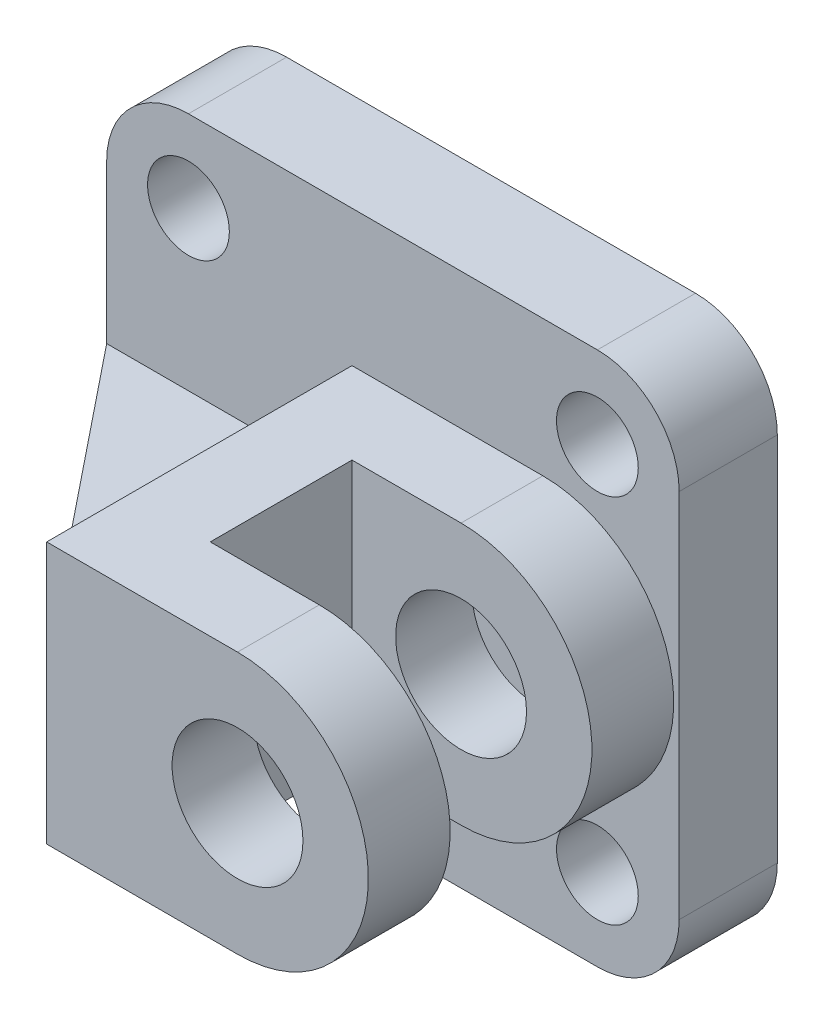
ISO-10303-21;
HEADER;
FILE_DESCRIPTION(('STEP AP214'),'2;1');
FILE_NAME('part.step','',(''),(''),'','','');
FILE_SCHEMA(('AUTOMOTIVE_DESIGN { 1 0 10303 214 1 1 1 1 }'));
ENDSEC;
DATA;
#1=APPLICATION_CONTEXT('core data for automotive mechanical design processes');
#2=APPLICATION_PROTOCOL_DEFINITION('international standard','automotive_design',2000,#1);
#3=PRODUCT_CONTEXT('',#1,'mechanical');
#4=PRODUCT('Part','Part','',(#3));
#5=PRODUCT_RELATED_PRODUCT_CATEGORY('part','',(#4));
#6=PRODUCT_DEFINITION_FORMATION('','',#4);
#7=PRODUCT_DEFINITION_CONTEXT('part definition',#1,'design');
#8=PRODUCT_DEFINITION('design','',#6,#7);
#9=PRODUCT_DEFINITION_SHAPE('','',#8);
#10=(LENGTH_UNIT() NAMED_UNIT(*) SI_UNIT(.MILLI.,.METRE.));
#11=(NAMED_UNIT(*) PLANE_ANGLE_UNIT() SI_UNIT($,.RADIAN.));
#12=(NAMED_UNIT(*) SI_UNIT($,.STERADIAN.) SOLID_ANGLE_UNIT());
#13=UNCERTAINTY_MEASURE_WITH_UNIT(LENGTH_MEASURE(1.E-05),#10,'distance_accuracy_value','');
#14=(GEOMETRIC_REPRESENTATION_CONTEXT(3) GLOBAL_UNCERTAINTY_ASSIGNED_CONTEXT((#13)) GLOBAL_UNIT_ASSIGNED_CONTEXT((#10,
#11,#12)) REPRESENTATION_CONTEXT('',''));
#15=CARTESIAN_POINT('',(0.,0.,0.));
#16=DIRECTION('',(0.,0.,1.));
#17=DIRECTION('',(1.,0.,0.));
#18=AXIS2_PLACEMENT_3D('',#15,#16,#17);
#19=CARTESIAN_POINT('',(0.,73.,18.));
#20=DIRECTION('',(-0.779508934793305,0.,0.626391108316048));
#21=DIRECTION('',(0.626391108316048,0.,0.779508934793305));
#22=AXIS2_PLACEMENT_3D('',#19,#20,#21);
#23=PLANE('',#22);
#24=DIRECTION('',(0.626391108316048,0.,0.779508934793305));
#25=VECTOR('',#24,1.);
#26=CARTESIAN_POINT('',(0.,54.,18.));
#27=LINE('',#26,#25);
#28=CARTESIAN_POINT('',(0.,54.,18.));
#29=VERTEX_POINT('',#28);
#30=CARTESIAN_POINT('',(45.,54.,74.));
#31=VERTEX_POINT('',#30);
#32=EDGE_CURVE('E64',#29,#31,#27,.T.);
#33=ORIENTED_EDGE('',*,*,#32,.F.);
#34=DIRECTION('',(0.,-1.,0.));
#35=VECTOR('',#34,1.);
#36=CARTESIAN_POINT('',(0.,73.,18.));
#37=LINE('',#36,#35);
#38=CARTESIAN_POINT('',(0.,44.,18.));
#39=VERTEX_POINT('',#38);
#40=EDGE_CURVE('E211',#29,#39,#37,.T.);
#41=ORIENTED_EDGE('',*,*,#40,.T.);
#42=DIRECTION('',(-0.626391108316048,0.,-0.779508934793305));
#43=VECTOR('',#42,1.);
#44=CARTESIAN_POINT('',(0.,44.,18.));
#45=LINE('',#44,#43);
#46=CARTESIAN_POINT('',(45.,44.,74.));
#47=VERTEX_POINT('',#46);
#48=EDGE_CURVE('E199',#47,#39,#45,.T.);
#49=ORIENTED_EDGE('',*,*,#48,.F.);
#50=DIRECTION('',(0.,-1.,0.));
#51=VECTOR('',#50,1.);
#52=CARTESIAN_POINT('',(45.,73.,74.));
#53=LINE('',#52,#51);
#54=EDGE_CURVE('E68',#31,#47,#53,.T.);
#55=ORIENTED_EDGE('',*,*,#54,.F.);
#56=EDGE_LOOP('',(#33,#41,#49,#55));
#57=FACE_BOUND('',#56,.T.);
#58=ADVANCED_FACE('F44',(#57),#23,.T.);
#59=CARTESIAN_POINT('',(15.,15.,18.));
#60=DIRECTION('',(0.,0.,-1.));
#61=DIRECTION('',(-1.,0.,0.));
#62=AXIS2_PLACEMENT_3D('',#59,#60,#61);
#63=PLANE('',#62);
#64=CARTESIAN_POINT('',(15.,15.,18.));
#65=DIRECTION('',(0.,0.,1.));
#66=DIRECTION('',(1.,0.,0.));
#67=AXIS2_PLACEMENT_3D('',#64,#65,#66);
#68=CIRCLE('',#67,7.5);
#69=CARTESIAN_POINT('',(22.5,15.,18.));
#70=VERTEX_POINT('',#69);
#71=EDGE_CURVE('E280',#70,#70,#68,.T.);
#72=ORIENTED_EDGE('',*,*,#71,.F.);
#73=EDGE_LOOP('',(#72));
#74=FACE_BOUND('',#73,.T.);
#75=CARTESIAN_POINT('',(90.,15.,18.));
#76=DIRECTION('',(0.,0.,1.));
#77=DIRECTION('',(1.,0.,0.));
#78=AXIS2_PLACEMENT_3D('',#75,#76,#77);
#79=CIRCLE('',#78,7.5);
#80=CARTESIAN_POINT('',(97.5,15.,18.));
#81=VERTEX_POINT('',#80);
#82=EDGE_CURVE('E286',#81,#81,#79,.T.);
#83=ORIENTED_EDGE('',*,*,#82,.F.);
#84=EDGE_LOOP('',(#83));
#85=FACE_BOUND('',#84,.T.);
#86=CARTESIAN_POINT('',(90.,83.,18.));
#87=DIRECTION('',(0.,0.,1.));
#88=DIRECTION('',(1.,0.,0.));
#89=AXIS2_PLACEMENT_3D('',#86,#87,#88);
#90=CIRCLE('',#89,7.5);
#91=CARTESIAN_POINT('',(97.5,83.,18.));
#92=VERTEX_POINT('',#91);
#93=EDGE_CURVE('E282',#92,#92,#90,.T.);
#94=ORIENTED_EDGE('',*,*,#93,.F.);
#95=EDGE_LOOP('',(#94));
#96=FACE_BOUND('',#95,.T.);
#97=CARTESIAN_POINT('',(15.,83.,18.));
#98=DIRECTION('',(0.,0.,1.));
#99=DIRECTION('',(1.,0.,0.));
#100=AXIS2_PLACEMENT_3D('',#97,#98,#99);
#101=CIRCLE('',#100,7.49999999999999);
#102=CARTESIAN_POINT('',(22.5,83.,18.));
#103=VERTEX_POINT('',#102);
#104=EDGE_CURVE('E285',#103,#103,#101,.T.);
#105=ORIENTED_EDGE('',*,*,#104,.F.);
#106=EDGE_LOOP('',(#105));
#107=FACE_BOUND('',#106,.T.);
#108=DIRECTION('',(0.,-1.,0.));
#109=VECTOR('',#108,1.);
#110=CARTESIAN_POINT('',(0.,82.9999999999999,18.));
#111=LINE('',#110,#109);
#112=CARTESIAN_POINT('',(0.,82.9999999999999,18.));
#113=VERTEX_POINT('',#112);
#114=EDGE_CURVE('E192',#113,#29,#111,.T.);
#115=ORIENTED_EDGE('',*,*,#114,.T.);
#116=DIRECTION('',(-1.,0.,0.));
#117=VECTOR('',#116,1.);
#118=CARTESIAN_POINT('',(45.,54.,18.));
#119=LINE('',#118,#117);
#120=CARTESIAN_POINT('',(45.,54.,18.));
#121=VERTEX_POINT('',#120);
#122=EDGE_CURVE('E186',#121,#29,#119,.T.);
#123=ORIENTED_EDGE('',*,*,#122,.F.);
#124=DIRECTION('',(0.,1.,0.));
#125=VECTOR('',#124,1.);
#126=CARTESIAN_POINT('',(45.,54.,18.));
#127=LINE('',#126,#125);
#128=CARTESIAN_POINT('',(45.,73.,18.));
#129=VERTEX_POINT('',#128);
#130=EDGE_CURVE('E179',#121,#129,#127,.T.);
#131=ORIENTED_EDGE('',*,*,#130,.T.);
#132=DIRECTION('',(-1.,0.,0.));
#133=VECTOR('',#132,1.);
#134=CARTESIAN_POINT('',(80.,73.,18.));
#135=LINE('',#134,#133);
#136=CARTESIAN_POINT('',(80.,73.,18.));
#137=VERTEX_POINT('',#136);
#138=EDGE_CURVE('E268',#137,#129,#135,.T.);
#139=ORIENTED_EDGE('',*,*,#138,.F.);
#140=CARTESIAN_POINT('',(80.,49.,18.));
#141=DIRECTION('',(0.,0.,1.));
#142=DIRECTION('',(1.,0.,0.));
#143=AXIS2_PLACEMENT_3D('',#140,#141,#142);
#144=CIRCLE('',#143,24.);
#145=CARTESIAN_POINT('',(80.,25.,18.));
#146=VERTEX_POINT('',#145);
#147=EDGE_CURVE('E256',#146,#137,#144,.T.);
#148=ORIENTED_EDGE('',*,*,#147,.F.);
#149=DIRECTION('',(1.,0.,0.));
#150=VECTOR('',#149,1.);
#151=CARTESIAN_POINT('',(45.,25.,18.));
#152=LINE('',#151,#150);
#153=CARTESIAN_POINT('',(45.,25.,18.));
#154=VERTEX_POINT('',#153);
#155=EDGE_CURVE('E265',#154,#146,#152,.T.);
#156=ORIENTED_EDGE('',*,*,#155,.F.);
#157=DIRECTION('',(0.,-1.,0.));
#158=VECTOR('',#157,1.);
#159=CARTESIAN_POINT('',(45.,44.,18.));
#160=LINE('',#159,#158);
#161=CARTESIAN_POINT('',(45.,44.,18.));
#162=VERTEX_POINT('',#161);
#163=EDGE_CURVE('E206',#162,#154,#160,.T.);
#164=ORIENTED_EDGE('',*,*,#163,.F.);
#165=DIRECTION('',(1.,0.,0.));
#166=VECTOR('',#165,1.);
#167=CARTESIAN_POINT('',(45.,44.,18.));
#168=LINE('',#167,#166);
#169=EDGE_CURVE('E205',#39,#162,#168,.T.);
#170=ORIENTED_EDGE('',*,*,#169,.F.);
#171=CARTESIAN_POINT('',(0.,15.0000000000001,18.));
#172=VERTEX_POINT('',#171);
#173=EDGE_CURVE('E316',#39,#172,#111,.T.);
#174=ORIENTED_EDGE('',*,*,#173,.T.);
#175=CARTESIAN_POINT('',(15.,15.,18.));
#176=DIRECTION('',(0.,0.,1.));
#177=DIRECTION('',(-1.,0.,0.));
#178=AXIS2_PLACEMENT_3D('',#175,#176,#177);
#179=CIRCLE('',#178,15.);
#180=CARTESIAN_POINT('',(15.0000000000001,0.,18.));
#181=VERTEX_POINT('',#180);
#182=EDGE_CURVE('E303',#172,#181,#179,.T.);
#183=ORIENTED_EDGE('',*,*,#182,.T.);
#184=DIRECTION('',(1.,0.,0.));
#185=VECTOR('',#184,1.);
#186=CARTESIAN_POINT('',(15.0000000000001,0.,18.));
#187=LINE('',#186,#185);
#188=CARTESIAN_POINT('',(89.9999999999999,0.,18.));
#189=VERTEX_POINT('',#188);
#190=EDGE_CURVE('E306',#181,#189,#187,.T.);
#191=ORIENTED_EDGE('',*,*,#190,.T.);
#192=CARTESIAN_POINT('',(90.,15.,18.));
#193=DIRECTION('',(0.,0.,1.));
#194=DIRECTION('',(-1.,0.,0.));
#195=AXIS2_PLACEMENT_3D('',#192,#193,#194);
#196=CIRCLE('',#195,15.);
#197=CARTESIAN_POINT('',(105.,15.0000000000001,18.));
#198=VERTEX_POINT('',#197);
#199=EDGE_CURVE('E307',#189,#198,#196,.T.);
#200=ORIENTED_EDGE('',*,*,#199,.T.);
#201=DIRECTION('',(0.,1.,0.));
#202=VECTOR('',#201,1.);
#203=CARTESIAN_POINT('',(105.,15.0000000000001,18.));
#204=LINE('',#203,#202);
#205=CARTESIAN_POINT('',(105.,82.9999999999999,18.));
#206=VERTEX_POINT('',#205);
#207=EDGE_CURVE('E311',#198,#206,#204,.T.);
#208=ORIENTED_EDGE('',*,*,#207,.T.);
#209=CARTESIAN_POINT('',(90.,83.,18.));
#210=DIRECTION('',(0.,0.,1.));
#211=DIRECTION('',(1.,0.,0.));
#212=AXIS2_PLACEMENT_3D('',#209,#210,#211);
#213=CIRCLE('',#212,15.);
#214=CARTESIAN_POINT('',(89.9999999999999,98.,18.));
#215=VERTEX_POINT('',#214);
#216=EDGE_CURVE('E312',#206,#215,#213,.T.);
#217=ORIENTED_EDGE('',*,*,#216,.T.);
#218=DIRECTION('',(-1.,0.,0.));
#219=VECTOR('',#218,1.);
#220=CARTESIAN_POINT('',(89.9999999999999,98.,18.));
#221=LINE('',#220,#219);
#222=CARTESIAN_POINT('',(15.0000000000001,98.,18.));
#223=VERTEX_POINT('',#222);
#224=EDGE_CURVE('E314',#215,#223,#221,.T.);
#225=ORIENTED_EDGE('',*,*,#224,.T.);
#226=CARTESIAN_POINT('',(15.,83.,18.));
#227=DIRECTION('',(0.,0.,1.));
#228=DIRECTION('',(-1.,0.,0.));
#229=AXIS2_PLACEMENT_3D('',#226,#227,#228);
#230=CIRCLE('',#229,15.);
#231=EDGE_CURVE('E320',#223,#113,#230,.T.);
#232=ORIENTED_EDGE('',*,*,#231,.T.);
#233=EDGE_LOOP('',(#115,#123,#131,#139,#148,#156,#164,#170,#174,#183,#191,#200,#208,#217,#225,#232));
#234=FACE_BOUND('',#233,.T.);
#235=ADVANCED_FACE('F195',(#74,#85,#96,#107,#234),#63,.F.);
#236=CARTESIAN_POINT('',(80.,49.,33.));
#237=DIRECTION('',(0.,0.,1.));
#238=DIRECTION('',(1.,0.,0.));
#239=AXIS2_PLACEMENT_3D('',#236,#237,#238);
#240=PLANE('',#239);
#241=CARTESIAN_POINT('',(80.,49.,33.));
#242=DIRECTION('',(0.,0.,1.));
#243=DIRECTION('',(1.,0.,0.));
#244=AXIS2_PLACEMENT_3D('',#241,#242,#243);
#245=CIRCLE('',#244,12.);
#246=CARTESIAN_POINT('',(92.,49.,33.));
#247=VERTEX_POINT('',#246);
#248=EDGE_CURVE('E222',#247,#247,#245,.T.);
#249=ORIENTED_EDGE('',*,*,#248,.F.);
#250=EDGE_LOOP('',(#249));
#251=FACE_BOUND('',#250,.T.);
#252=DIRECTION('',(0.,1.,0.));
#253=VECTOR('',#252,1.);
#254=CARTESIAN_POINT('',(60.,25.,33.));
#255=LINE('',#254,#253);
#256=CARTESIAN_POINT('',(60.,25.,33.));
#257=VERTEX_POINT('',#256);
#258=CARTESIAN_POINT('',(60.,73.,33.));
#259=VERTEX_POINT('',#258);
#260=EDGE_CURVE('E250',#257,#259,#255,.T.);
#261=ORIENTED_EDGE('',*,*,#260,.F.);
#262=DIRECTION('',(1.,0.,0.));
#263=VECTOR('',#262,1.);
#264=CARTESIAN_POINT('',(45.,25.,33.));
#265=LINE('',#264,#263);
#266=CARTESIAN_POINT('',(80.,25.,33.));
#267=VERTEX_POINT('',#266);
#268=EDGE_CURVE('E264',#257,#267,#265,.T.);
#269=ORIENTED_EDGE('',*,*,#268,.T.);
#270=CARTESIAN_POINT('',(80.,49.,33.));
#271=DIRECTION('',(0.,0.,1.));
#272=DIRECTION('',(1.,0.,0.));
#273=AXIS2_PLACEMENT_3D('',#270,#271,#272);
#274=CIRCLE('',#273,24.);
#275=CARTESIAN_POINT('',(80.,73.,33.));
#276=VERTEX_POINT('',#275);
#277=EDGE_CURVE('E260',#267,#276,#274,.T.);
#278=ORIENTED_EDGE('',*,*,#277,.T.);
#279=DIRECTION('',(-1.,0.,0.));
#280=VECTOR('',#279,1.);
#281=CARTESIAN_POINT('',(80.,73.,33.));
#282=LINE('',#281,#280);
#283=EDGE_CURVE('E261',#276,#259,#282,.T.);
#284=ORIENTED_EDGE('',*,*,#283,.T.);
#285=EDGE_LOOP('',(#261,#269,#278,#284));
#286=FACE_BOUND('',#285,.T.);
#287=ADVANCED_FACE('F415',(#251,#286),#240,.T.);
#288=CARTESIAN_POINT('',(15.,15.,18.));
#289=DIRECTION('',(0.,0.,-1.));
#290=DIRECTION('',(-1.,0.,0.));
#291=AXIS2_PLACEMENT_3D('',#288,#289,#290);
#292=CYLINDRICAL_SURFACE('',#291,15.);
#293=CARTESIAN_POINT('',(15.,15.,0.));
#294=DIRECTION('',(0.,0.,1.));
#295=DIRECTION('',(-1.,0.,0.));
#296=AXIS2_PLACEMENT_3D('',#293,#294,#295);
#297=CIRCLE('',#296,15.);
#298=CARTESIAN_POINT('',(0.,15.0000000000001,0.));
#299=VERTEX_POINT('',#298);
#300=CARTESIAN_POINT('',(15.0000000000001,0.,0.));
#301=VERTEX_POINT('',#300);
#302=EDGE_CURVE('E297',#299,#301,#297,.T.);
#303=ORIENTED_EDGE('',*,*,#302,.T.);
#304=DIRECTION('',(0.,0.,-1.));
#305=VECTOR('',#304,1.);
#306=CARTESIAN_POINT('',(15.0000000000001,0.,18.));
#307=LINE('',#306,#305);
#308=EDGE_CURVE('E11',#181,#301,#307,.T.);
#309=ORIENTED_EDGE('',*,*,#308,.F.);
#310=ORIENTED_EDGE('',*,*,#182,.F.);
#311=DIRECTION('',(0.,0.,-1.));
#312=VECTOR('',#311,1.);
#313=CARTESIAN_POINT('',(0.,15.0000000000001,18.));
#314=LINE('',#313,#312);
#315=EDGE_CURVE('E324',#172,#299,#314,.T.);
#316=ORIENTED_EDGE('',*,*,#315,.T.);
#317=EDGE_LOOP('',(#303,#309,#310,#316));
#318=FACE_BOUND('',#317,.T.);
#319=ADVANCED_FACE('F50',(#318),#292,.T.);
#320=CARTESIAN_POINT('',(15.0000000000001,0.,18.));
#321=DIRECTION('',(0.,1.,0.));
#322=DIRECTION('',(0.,0.,1.));
#323=AXIS2_PLACEMENT_3D('',#320,#321,#322);
#324=PLANE('',#323);
#325=DIRECTION('',(1.,0.,0.));
#326=VECTOR('',#325,1.);
#327=CARTESIAN_POINT('',(15.0000000000001,0.,0.));
#328=LINE('',#327,#326);
#329=CARTESIAN_POINT('',(89.9999999999999,0.,0.));
#330=VERTEX_POINT('',#329);
#331=EDGE_CURVE('E323',#301,#330,#328,.T.);
#332=ORIENTED_EDGE('',*,*,#331,.T.);
#333=DIRECTION('',(0.,0.,-1.));
#334=VECTOR('',#333,1.);
#335=CARTESIAN_POINT('',(89.9999999999999,0.,18.));
#336=LINE('',#335,#334);
#337=EDGE_CURVE('E53',#189,#330,#336,.T.);
#338=ORIENTED_EDGE('',*,*,#337,.F.);
#339=ORIENTED_EDGE('',*,*,#190,.F.);
#340=ORIENTED_EDGE('',*,*,#308,.T.);
#341=EDGE_LOOP('',(#332,#338,#339,#340));
#342=FACE_BOUND('',#341,.T.);
#343=ADVANCED_FACE('F379',(#342),#324,.F.);
#344=CARTESIAN_POINT('',(90.,15.,18.));
#345=DIRECTION('',(0.,0.,-1.));
#346=DIRECTION('',(-1.,0.,0.));
#347=AXIS2_PLACEMENT_3D('',#344,#345,#346);
#348=CYLINDRICAL_SURFACE('',#347,15.);
#349=CARTESIAN_POINT('',(90.,15.,0.));
#350=DIRECTION('',(0.,0.,1.));
#351=DIRECTION('',(-1.,0.,0.));
#352=AXIS2_PLACEMENT_3D('',#349,#350,#351);
#353=CIRCLE('',#352,15.);
#354=CARTESIAN_POINT('',(105.,15.0000000000001,0.));
#355=VERTEX_POINT('',#354);
#356=EDGE_CURVE('E326',#330,#355,#353,.T.);
#357=ORIENTED_EDGE('',*,*,#356,.T.);
#358=DIRECTION('',(0.,0.,-1.));
#359=VECTOR('',#358,1.);
#360=CARTESIAN_POINT('',(105.,15.0000000000001,18.));
#361=LINE('',#360,#359);
#362=EDGE_CURVE('E352',#198,#355,#361,.T.);
#363=ORIENTED_EDGE('',*,*,#362,.F.);
#364=ORIENTED_EDGE('',*,*,#199,.F.);
#365=ORIENTED_EDGE('',*,*,#337,.T.);
#366=EDGE_LOOP('',(#357,#363,#364,#365));
#367=FACE_BOUND('',#366,.T.);
#368=ADVANCED_FACE('F360',(#367),#348,.T.);
#369=CARTESIAN_POINT('',(105.,15.0000000000001,18.));
#370=DIRECTION('',(-1.,0.,0.));
#371=DIRECTION('',(0.,0.,1.));
#372=AXIS2_PLACEMENT_3D('',#369,#370,#371);
#373=PLANE('',#372);
#374=DIRECTION('',(0.,1.,0.));
#375=VECTOR('',#374,1.);
#376=CARTESIAN_POINT('',(105.,15.0000000000001,0.));
#377=LINE('',#376,#375);
#378=CARTESIAN_POINT('',(105.,82.9999999999999,0.));
#379=VERTEX_POINT('',#378);
#380=EDGE_CURVE('E327',#355,#379,#377,.T.);
#381=ORIENTED_EDGE('',*,*,#380,.T.);
#382=DIRECTION('',(0.,0.,-1.));
#383=VECTOR('',#382,1.);
#384=CARTESIAN_POINT('',(105.,82.9999999999999,18.));
#385=LINE('',#384,#383);
#386=EDGE_CURVE('E347',#206,#379,#385,.T.);
#387=ORIENTED_EDGE('',*,*,#386,.F.);
#388=ORIENTED_EDGE('',*,*,#207,.F.);
#389=ORIENTED_EDGE('',*,*,#362,.T.);
#390=EDGE_LOOP('',(#381,#387,#388,#389));
#391=FACE_BOUND('',#390,.T.);
#392=ADVANCED_FACE('F369',(#391),#373,.F.);
#393=CARTESIAN_POINT('',(90.,83.,18.));
#394=DIRECTION('',(0.,0.,-1.));
#395=DIRECTION('',(-1.,0.,0.));
#396=AXIS2_PLACEMENT_3D('',#393,#394,#395);
#397=CYLINDRICAL_SURFACE('',#396,15.);
#398=CARTESIAN_POINT('',(90.,83.,0.));
#399=DIRECTION('',(0.,0.,1.));
#400=DIRECTION('',(1.,0.,0.));
#401=AXIS2_PLACEMENT_3D('',#398,#399,#400);
#402=CIRCLE('',#401,15.);
#403=CARTESIAN_POINT('',(89.9999999999999,98.,0.));
#404=VERTEX_POINT('',#403);
#405=EDGE_CURVE('E329',#379,#404,#402,.T.);
#406=ORIENTED_EDGE('',*,*,#405,.T.);
#407=DIRECTION('',(0.,0.,-1.));
#408=VECTOR('',#407,1.);
#409=CARTESIAN_POINT('',(89.9999999999999,98.,18.));
#410=LINE('',#409,#408);
#411=EDGE_CURVE('E342',#215,#404,#410,.T.);
#412=ORIENTED_EDGE('',*,*,#411,.F.);
#413=ORIENTED_EDGE('',*,*,#216,.F.);
#414=ORIENTED_EDGE('',*,*,#386,.T.);
#415=EDGE_LOOP('',(#406,#412,#413,#414));
#416=FACE_BOUND('',#415,.T.);
#417=ADVANCED_FACE('F372',(#416),#397,.T.);
#418=CARTESIAN_POINT('',(89.9999999999999,98.,18.));
#419=DIRECTION('',(0.,-1.,0.));
#420=DIRECTION('',(0.,0.,-1.));
#421=AXIS2_PLACEMENT_3D('',#418,#419,#420);
#422=PLANE('',#421);
#423=DIRECTION('',(-1.,0.,0.));
#424=VECTOR('',#423,1.);
#425=CARTESIAN_POINT('',(89.9999999999999,98.,0.));
#426=LINE('',#425,#424);
#427=CARTESIAN_POINT('',(15.0000000000001,98.,0.));
#428=VERTEX_POINT('',#427);
#429=EDGE_CURVE('E334',#404,#428,#426,.T.);
#430=ORIENTED_EDGE('',*,*,#429,.T.);
#431=DIRECTION('',(0.,0.,-1.));
#432=VECTOR('',#431,1.);
#433=CARTESIAN_POINT('',(15.0000000000001,98.,18.));
#434=LINE('',#433,#432);
#435=EDGE_CURVE('E341',#223,#428,#434,.T.);
#436=ORIENTED_EDGE('',*,*,#435,.F.);
#437=ORIENTED_EDGE('',*,*,#224,.F.);
#438=ORIENTED_EDGE('',*,*,#411,.T.);
#439=EDGE_LOOP('',(#430,#436,#437,#438));
#440=FACE_BOUND('',#439,.T.);
#441=ADVANCED_FACE('F393',(#440),#422,.F.);
#442=CARTESIAN_POINT('',(15.,83.,18.));
#443=DIRECTION('',(0.,0.,-1.));
#444=DIRECTION('',(-1.,0.,0.));
#445=AXIS2_PLACEMENT_3D('',#442,#443,#444);
#446=CYLINDRICAL_SURFACE('',#445,15.);
#447=CARTESIAN_POINT('',(15.,83.,0.));
#448=DIRECTION('',(0.,0.,1.));
#449=DIRECTION('',(-1.,0.,0.));
#450=AXIS2_PLACEMENT_3D('',#447,#448,#449);
#451=CIRCLE('',#450,15.);
#452=CARTESIAN_POINT('',(0.,82.9999999999999,0.));
#453=VERTEX_POINT('',#452);
#454=EDGE_CURVE('E331',#428,#453,#451,.T.);
#455=ORIENTED_EDGE('',*,*,#454,.T.);
#456=DIRECTION('',(0.,0.,-1.));
#457=VECTOR('',#456,1.);
#458=CARTESIAN_POINT('',(0.,82.9999999999999,18.));
#459=LINE('',#458,#457);
#460=EDGE_CURVE('E339',#113,#453,#459,.T.);
#461=ORIENTED_EDGE('',*,*,#460,.F.);
#462=ORIENTED_EDGE('',*,*,#231,.F.);
#463=ORIENTED_EDGE('',*,*,#435,.T.);
#464=EDGE_LOOP('',(#455,#461,#462,#463));
#465=FACE_BOUND('',#464,.T.);
#466=ADVANCED_FACE('F395',(#465),#446,.T.);
#467=CARTESIAN_POINT('',(0.,82.9999999999999,18.));
#468=DIRECTION('',(1.,0.,0.));
#469=DIRECTION('',(0.,0.,-1.));
#470=AXIS2_PLACEMENT_3D('',#467,#468,#469);
#471=PLANE('',#470);
#472=DIRECTION('',(0.,-1.,0.));
#473=VECTOR('',#472,1.);
#474=CARTESIAN_POINT('',(0.,82.9999999999999,0.));
#475=LINE('',#474,#473);
#476=EDGE_CURVE('E310',#453,#299,#475,.T.);
#477=ORIENTED_EDGE('',*,*,#476,.T.);
#478=ORIENTED_EDGE('',*,*,#315,.F.);
#479=ORIENTED_EDGE('',*,*,#173,.F.);
#480=ORIENTED_EDGE('',*,*,#40,.F.);
#481=ORIENTED_EDGE('',*,*,#114,.F.);
#482=ORIENTED_EDGE('',*,*,#460,.T.);
#483=EDGE_LOOP('',(#477,#478,#479,#480,#481,#482));
#484=FACE_BOUND('',#483,.T.);
#485=ADVANCED_FACE('F389',(#484),#471,.F.);
#486=CARTESIAN_POINT('',(15.,15.,0.));
#487=DIRECTION('',(0.,0.,-1.));
#488=DIRECTION('',(-1.,0.,0.));
#489=AXIS2_PLACEMENT_3D('',#486,#487,#488);
#490=PLANE('',#489);
#491=CARTESIAN_POINT('',(15.,15.,0.));
#492=DIRECTION('',(0.,0.,1.));
#493=DIRECTION('',(1.,0.,0.));
#494=AXIS2_PLACEMENT_3D('',#491,#492,#493);
#495=CIRCLE('',#494,7.5);
#496=CARTESIAN_POINT('',(22.5,15.,0.));
#497=VERTEX_POINT('',#496);
#498=EDGE_CURVE('E292',#497,#497,#495,.T.);
#499=ORIENTED_EDGE('',*,*,#498,.T.);
#500=EDGE_LOOP('',(#499));
#501=FACE_BOUND('',#500,.T.);
#502=CARTESIAN_POINT('',(90.,15.,0.));
#503=DIRECTION('',(0.,0.,1.));
#504=DIRECTION('',(1.,0.,0.));
#505=AXIS2_PLACEMENT_3D('',#502,#503,#504);
#506=CIRCLE('',#505,7.5);
#507=CARTESIAN_POINT('',(97.5,15.,0.));
#508=VERTEX_POINT('',#507);
#509=EDGE_CURVE('E287',#508,#508,#506,.T.);
#510=ORIENTED_EDGE('',*,*,#509,.T.);
#511=EDGE_LOOP('',(#510));
#512=FACE_BOUND('',#511,.T.);
#513=CARTESIAN_POINT('',(90.,83.,0.));
#514=DIRECTION('',(0.,0.,1.));
#515=DIRECTION('',(1.,0.,0.));
#516=AXIS2_PLACEMENT_3D('',#513,#514,#515);
#517=CIRCLE('',#516,7.5);
#518=CARTESIAN_POINT('',(97.5,83.,0.));
#519=VERTEX_POINT('',#518);
#520=EDGE_CURVE('E278',#519,#519,#517,.T.);
#521=ORIENTED_EDGE('',*,*,#520,.T.);
#522=EDGE_LOOP('',(#521));
#523=FACE_BOUND('',#522,.T.);
#524=CARTESIAN_POINT('',(15.,83.,0.));
#525=DIRECTION('',(0.,0.,1.));
#526=DIRECTION('',(1.,0.,0.));
#527=AXIS2_PLACEMENT_3D('',#524,#525,#526);
#528=CIRCLE('',#527,7.49999999999999);
#529=CARTESIAN_POINT('',(22.5,83.,0.));
#530=VERTEX_POINT('',#529);
#531=EDGE_CURVE('E300',#530,#530,#528,.T.);
#532=ORIENTED_EDGE('',*,*,#531,.T.);
#533=EDGE_LOOP('',(#532));
#534=FACE_BOUND('',#533,.T.);
#535=ORIENTED_EDGE('',*,*,#302,.F.);
#536=ORIENTED_EDGE('',*,*,#476,.F.);
#537=ORIENTED_EDGE('',*,*,#454,.F.);
#538=ORIENTED_EDGE('',*,*,#429,.F.);
#539=ORIENTED_EDGE('',*,*,#405,.F.);
#540=ORIENTED_EDGE('',*,*,#380,.F.);
#541=ORIENTED_EDGE('',*,*,#356,.F.);
#542=ORIENTED_EDGE('',*,*,#331,.F.);
#543=EDGE_LOOP('',(#535,#536,#537,#538,#539,#540,#541,#542));
#544=FACE_BOUND('',#543,.T.);
#545=ADVANCED_FACE('F362',(#501,#512,#523,#534,#544),#490,.T.);
#546=CARTESIAN_POINT('',(15.,83.,0.));
#547=DIRECTION('',(0.,0.,1.));
#548=DIRECTION('',(1.,0.,0.));
#549=AXIS2_PLACEMENT_3D('',#546,#547,#548);
#550=CYLINDRICAL_SURFACE('',#549,7.49999999999999);
#551=ORIENTED_EDGE('',*,*,#531,.F.);
#552=EDGE_LOOP('',(#551));
#553=FACE_BOUND('',#552,.T.);
#554=ORIENTED_EDGE('',*,*,#104,.T.);
#555=EDGE_LOOP('',(#554));
#556=FACE_BOUND('',#555,.T.);
#557=ADVANCED_FACE('F461',(#553,#556),#550,.F.);
#558=CARTESIAN_POINT('',(90.,83.,0.));
#559=DIRECTION('',(0.,0.,1.));
#560=DIRECTION('',(1.,0.,0.));
#561=AXIS2_PLACEMENT_3D('',#558,#559,#560);
#562=CYLINDRICAL_SURFACE('',#561,7.5);
#563=ORIENTED_EDGE('',*,*,#520,.F.);
#564=EDGE_LOOP('',(#563));
#565=FACE_BOUND('',#564,.T.);
#566=ORIENTED_EDGE('',*,*,#93,.T.);
#567=EDGE_LOOP('',(#566));
#568=FACE_BOUND('',#567,.T.);
#569=ADVANCED_FACE('F459',(#565,#568),#562,.F.);
#570=CARTESIAN_POINT('',(90.,15.,0.));
#571=DIRECTION('',(0.,0.,1.));
#572=DIRECTION('',(1.,0.,0.));
#573=AXIS2_PLACEMENT_3D('',#570,#571,#572);
#574=CYLINDRICAL_SURFACE('',#573,7.5);
#575=ORIENTED_EDGE('',*,*,#509,.F.);
#576=EDGE_LOOP('',(#575));
#577=FACE_BOUND('',#576,.T.);
#578=ORIENTED_EDGE('',*,*,#82,.T.);
#579=EDGE_LOOP('',(#578));
#580=FACE_BOUND('',#579,.T.);
#581=ADVANCED_FACE('F465',(#577,#580),#574,.F.);
#582=CARTESIAN_POINT('',(15.,15.,0.));
#583=DIRECTION('',(0.,0.,1.));
#584=DIRECTION('',(1.,0.,0.));
#585=AXIS2_PLACEMENT_3D('',#582,#583,#584);
#586=CYLINDRICAL_SURFACE('',#585,7.5);
#587=ORIENTED_EDGE('',*,*,#498,.F.);
#588=EDGE_LOOP('',(#587));
#589=FACE_BOUND('',#588,.T.);
#590=ORIENTED_EDGE('',*,*,#71,.T.);
#591=EDGE_LOOP('',(#590));
#592=FACE_BOUND('',#591,.T.);
#593=ADVANCED_FACE('F457',(#589,#592),#586,.F.);
#594=CARTESIAN_POINT('',(80.,49.,33.));
#595=DIRECTION('',(0.,0.,-1.));
#596=DIRECTION('',(-1.,0.,0.));
#597=AXIS2_PLACEMENT_3D('',#594,#595,#596);
#598=CYLINDRICAL_SURFACE('',#597,24.);
#599=ORIENTED_EDGE('',*,*,#147,.T.);
#600=DIRECTION('',(0.,0.,-1.));
#601=VECTOR('',#600,1.);
#602=CARTESIAN_POINT('',(80.,73.,33.));
#603=LINE('',#602,#601);
#604=EDGE_CURVE('E273',#276,#137,#603,.T.);
#605=ORIENTED_EDGE('',*,*,#604,.F.);
#606=ORIENTED_EDGE('',*,*,#277,.F.);
#607=DIRECTION('',(0.,0.,-1.));
#608=VECTOR('',#607,1.);
#609=CARTESIAN_POINT('',(80.,25.,33.));
#610=LINE('',#609,#608);
#611=EDGE_CURVE('E269',#267,#146,#610,.T.);
#612=ORIENTED_EDGE('',*,*,#611,.T.);
#613=EDGE_LOOP('',(#599,#605,#606,#612));
#614=FACE_BOUND('',#613,.T.);
#615=ADVANCED_FACE('F453',(#614),#598,.T.);
#616=CARTESIAN_POINT('',(80.,73.,33.));
#617=DIRECTION('',(0.,-1.,0.));
#618=DIRECTION('',(0.,0.,-1.));
#619=AXIS2_PLACEMENT_3D('',#616,#617,#618);
#620=PLANE('',#619);
#621=ORIENTED_EDGE('',*,*,#138,.T.);
#622=DIRECTION('',(0.,0.,-1.));
#623=VECTOR('',#622,1.);
#624=CARTESIAN_POINT('',(45.,73.,74.));
#625=LINE('',#624,#623);
#626=CARTESIAN_POINT('',(45.,73.,74.));
#627=VERTEX_POINT('',#626);
#628=EDGE_CURVE('E183',#627,#129,#625,.T.);
#629=ORIENTED_EDGE('',*,*,#628,.F.);
#630=DIRECTION('',(-1.,0.,0.));
#631=VECTOR('',#630,1.);
#632=CARTESIAN_POINT('',(45.,73.,74.));
#633=LINE('',#632,#631);
#634=CARTESIAN_POINT('',(80.,73.,74.));
#635=VERTEX_POINT('',#634);
#636=EDGE_CURVE('E249',#635,#627,#633,.T.);
#637=ORIENTED_EDGE('',*,*,#636,.F.);
#638=DIRECTION('',(0.,0.,1.));
#639=VECTOR('',#638,1.);
#640=CARTESIAN_POINT('',(80.,73.,59.));
#641=LINE('',#640,#639);
#642=CARTESIAN_POINT('',(80.,73.,59.));
#643=VERTEX_POINT('',#642);
#644=EDGE_CURVE('E238',#643,#635,#641,.T.);
#645=ORIENTED_EDGE('',*,*,#644,.F.);
#646=DIRECTION('',(-1.,0.,0.));
#647=VECTOR('',#646,1.);
#648=CARTESIAN_POINT('',(60.,73.,59.));
#649=LINE('',#648,#647);
#650=CARTESIAN_POINT('',(60.,73.,59.));
#651=VERTEX_POINT('',#650);
#652=EDGE_CURVE('E234',#643,#651,#649,.T.);
#653=ORIENTED_EDGE('',*,*,#652,.T.);
#654=DIRECTION('',(0.,0.,1.));
#655=VECTOR('',#654,1.);
#656=CARTESIAN_POINT('',(60.,73.,33.));
#657=LINE('',#656,#655);
#658=EDGE_CURVE('E241',#259,#651,#657,.T.);
#659=ORIENTED_EDGE('',*,*,#658,.F.);
#660=ORIENTED_EDGE('',*,*,#283,.F.);
#661=ORIENTED_EDGE('',*,*,#604,.T.);
#662=EDGE_LOOP('',(#621,#629,#637,#645,#653,#659,#660,#661));
#663=FACE_BOUND('',#662,.T.);
#664=ADVANCED_FACE('F448',(#663),#620,.F.);
#665=CARTESIAN_POINT('',(45.,25.,33.));
#666=DIRECTION('',(0.,1.,0.));
#667=DIRECTION('',(0.,0.,1.));
#668=AXIS2_PLACEMENT_3D('',#665,#666,#667);
#669=PLANE('',#668);
#670=DIRECTION('',(-1.,0.,0.));
#671=VECTOR('',#670,1.);
#672=CARTESIAN_POINT('',(45.,25.,74.));
#673=LINE('',#672,#671);
#674=CARTESIAN_POINT('',(80.,25.,74.));
#675=VERTEX_POINT('',#674);
#676=CARTESIAN_POINT('',(45.,25.,74.));
#677=VERTEX_POINT('',#676);
#678=EDGE_CURVE('E248',#675,#677,#673,.T.);
#679=ORIENTED_EDGE('',*,*,#678,.T.);
#680=DIRECTION('',(0.,0.,1.));
#681=VECTOR('',#680,1.);
#682=CARTESIAN_POINT('',(45.,25.,74.));
#683=LINE('',#682,#681);
#684=EDGE_CURVE('E189',#154,#677,#683,.T.);
#685=ORIENTED_EDGE('',*,*,#684,.F.);
#686=ORIENTED_EDGE('',*,*,#155,.T.);
#687=ORIENTED_EDGE('',*,*,#611,.F.);
#688=ORIENTED_EDGE('',*,*,#268,.F.);
#689=DIRECTION('',(0.,0.,-1.));
#690=VECTOR('',#689,1.);
#691=CARTESIAN_POINT('',(60.,25.,74.));
#692=LINE('',#691,#690);
#693=CARTESIAN_POINT('',(60.,25.,59.));
#694=VERTEX_POINT('',#693);
#695=EDGE_CURVE('E244',#694,#257,#692,.T.);
#696=ORIENTED_EDGE('',*,*,#695,.F.);
#697=DIRECTION('',(1.,0.,0.));
#698=VECTOR('',#697,1.);
#699=CARTESIAN_POINT('',(80.,25.,59.));
#700=LINE('',#699,#698);
#701=CARTESIAN_POINT('',(80.,25.,59.));
#702=VERTEX_POINT('',#701);
#703=EDGE_CURVE('E235',#694,#702,#700,.T.);
#704=ORIENTED_EDGE('',*,*,#703,.T.);
#705=DIRECTION('',(0.,0.,1.));
#706=VECTOR('',#705,1.);
#707=CARTESIAN_POINT('',(80.,25.,59.));
#708=LINE('',#707,#706);
#709=EDGE_CURVE('E240',#702,#675,#708,.T.);
#710=ORIENTED_EDGE('',*,*,#709,.T.);
#711=EDGE_LOOP('',(#679,#685,#686,#687,#688,#696,#704,#710));
#712=FACE_BOUND('',#711,.T.);
#713=ADVANCED_FACE('F442',(#712),#669,.F.);
#714=CARTESIAN_POINT('',(45.,73.,74.));
#715=DIRECTION('',(0.,0.,1.));
#716=DIRECTION('',(1.,0.,0.));
#717=AXIS2_PLACEMENT_3D('',#714,#715,#716);
#718=PLANE('',#717);
#719=CARTESIAN_POINT('',(80.,49.,74.));
#720=DIRECTION('',(0.,0.,1.));
#721=DIRECTION('',(1.,0.,0.));
#722=AXIS2_PLACEMENT_3D('',#719,#720,#721);
#723=CIRCLE('',#722,12.);
#724=CARTESIAN_POINT('',(92.,49.,74.));
#725=VERTEX_POINT('',#724);
#726=EDGE_CURVE('E212',#725,#725,#723,.T.);
#727=ORIENTED_EDGE('',*,*,#726,.F.);
#728=EDGE_LOOP('',(#727));
#729=FACE_BOUND('',#728,.T.);
#730=ORIENTED_EDGE('',*,*,#678,.F.);
#731=CARTESIAN_POINT('',(80.,49.,74.));
#732=DIRECTION('',(0.,0.,1.));
#733=DIRECTION('',(1.,0.,0.));
#734=AXIS2_PLACEMENT_3D('',#731,#732,#733);
#735=CIRCLE('',#734,24.);
#736=EDGE_CURVE('E221',#675,#635,#735,.T.);
#737=ORIENTED_EDGE('',*,*,#736,.T.);
#738=ORIENTED_EDGE('',*,*,#636,.T.);
#739=EDGE_CURVE('E253',#627,#31,#53,.T.);
#740=ORIENTED_EDGE('',*,*,#739,.T.);
#741=ORIENTED_EDGE('',*,*,#54,.T.);
#742=DIRECTION('',(0.,-1.,0.));
#743=VECTOR('',#742,1.);
#744=CARTESIAN_POINT('',(45.,44.,74.));
#745=LINE('',#744,#743);
#746=EDGE_CURVE('E208',#47,#677,#745,.T.);
#747=ORIENTED_EDGE('',*,*,#746,.T.);
#748=EDGE_LOOP('',(#730,#737,#738,#740,#741,#747));
#749=FACE_BOUND('',#748,.T.);
#750=ADVANCED_FACE('F437',(#729,#749),#718,.T.);
#751=CARTESIAN_POINT('',(60.,0.,0.));
#752=DIRECTION('',(1.,0.,0.));
#753=DIRECTION('',(0.,0.,-1.));
#754=AXIS2_PLACEMENT_3D('',#751,#752,#753);
#755=PLANE('',#754);
#756=DIRECTION('',(0.,-1.,0.));
#757=VECTOR('',#756,1.);
#758=CARTESIAN_POINT('',(60.,25.,59.));
#759=LINE('',#758,#757);
#760=EDGE_CURVE('E226',#651,#694,#759,.T.);
#761=ORIENTED_EDGE('',*,*,#760,.T.);
#762=ORIENTED_EDGE('',*,*,#695,.T.);
#763=ORIENTED_EDGE('',*,*,#260,.T.);
#764=ORIENTED_EDGE('',*,*,#658,.T.);
#765=EDGE_LOOP('',(#761,#762,#763,#764));
#766=FACE_BOUND('',#765,.T.);
#767=ADVANCED_FACE('F434',(#766),#755,.T.);
#768=CARTESIAN_POINT('',(0.,0.,59.));
#769=DIRECTION('',(0.,0.,-1.));
#770=DIRECTION('',(-1.,0.,0.));
#771=AXIS2_PLACEMENT_3D('',#768,#769,#770);
#772=PLANE('',#771);
#773=CARTESIAN_POINT('',(80.,49.,59.));
#774=DIRECTION('',(0.,0.,-1.));
#775=DIRECTION('',(-1.,0.,0.));
#776=AXIS2_PLACEMENT_3D('',#773,#774,#775);
#777=CIRCLE('',#776,12.);
#778=CARTESIAN_POINT('',(68.,49.,59.));
#779=VERTEX_POINT('',#778);
#780=EDGE_CURVE('E47',#779,#779,#777,.T.);
#781=ORIENTED_EDGE('',*,*,#780,.F.);
#782=EDGE_LOOP('',(#781));
#783=FACE_BOUND('',#782,.T.);
#784=ORIENTED_EDGE('',*,*,#760,.F.);
#785=ORIENTED_EDGE('',*,*,#652,.F.);
#786=CARTESIAN_POINT('',(80.,49.,59.));
#787=DIRECTION('',(0.,0.,1.));
#788=DIRECTION('',(1.,0.,0.));
#789=AXIS2_PLACEMENT_3D('',#786,#787,#788);
#790=CIRCLE('',#789,24.);
#791=EDGE_CURVE('E223',#702,#643,#790,.T.);
#792=ORIENTED_EDGE('',*,*,#791,.F.);
#793=ORIENTED_EDGE('',*,*,#703,.F.);
#794=EDGE_LOOP('',(#784,#785,#792,#793));
#795=FACE_BOUND('',#794,.T.);
#796=ADVANCED_FACE('F431',(#783,#795),#772,.T.);
#797=CARTESIAN_POINT('',(80.,49.,59.));
#798=DIRECTION('',(0.,0.,1.));
#799=DIRECTION('',(1.,0.,0.));
#800=AXIS2_PLACEMENT_3D('',#797,#798,#799);
#801=CYLINDRICAL_SURFACE('',#800,24.);
#802=ORIENTED_EDGE('',*,*,#736,.F.);
#803=ORIENTED_EDGE('',*,*,#709,.F.);
#804=ORIENTED_EDGE('',*,*,#791,.T.);
#805=ORIENTED_EDGE('',*,*,#644,.T.);
#806=EDGE_LOOP('',(#802,#803,#804,#805));
#807=FACE_BOUND('',#806,.T.);
#808=ADVANCED_FACE('F430',(#807),#801,.T.);
#809=CARTESIAN_POINT('',(80.,49.,19.));
#810=DIRECTION('',(0.,0.,1.));
#811=DIRECTION('',(1.,0.,0.));
#812=AXIS2_PLACEMENT_3D('',#809,#810,#811);
#813=CYLINDRICAL_SURFACE('',#812,12.);
#814=ORIENTED_EDGE('',*,*,#780,.T.);
#815=EDGE_LOOP('',(#814));
#816=FACE_BOUND('',#815,.T.);
#817=ORIENTED_EDGE('',*,*,#726,.T.);
#818=EDGE_LOOP('',(#817));
#819=FACE_BOUND('',#818,.T.);
#820=ADVANCED_FACE('F425',(#816,#819),#813,.F.);
#821=ORIENTED_EDGE('',*,*,#248,.T.);
#822=EDGE_LOOP('',(#821));
#823=FACE_BOUND('',#822,.T.);
#824=CARTESIAN_POINT('',(80.,49.,19.));
#825=DIRECTION('',(0.,0.,1.));
#826=DIRECTION('',(1.,0.,0.));
#827=AXIS2_PLACEMENT_3D('',#824,#825,#826);
#828=CIRCLE('',#827,12.);
#829=CARTESIAN_POINT('',(92.,49.,19.));
#830=VERTEX_POINT('',#829);
#831=EDGE_CURVE('E216',#830,#830,#828,.T.);
#832=ORIENTED_EDGE('',*,*,#831,.F.);
#833=EDGE_LOOP('',(#832));
#834=FACE_BOUND('',#833,.T.);
#835=ADVANCED_FACE('F422',(#823,#834),#813,.F.);
#836=CARTESIAN_POINT('',(80.,49.,19.));
#837=DIRECTION('',(0.,0.,1.));
#838=DIRECTION('',(1.,0.,0.));
#839=AXIS2_PLACEMENT_3D('',#836,#837,#838);
#840=PLANE('',#839);
#841=ORIENTED_EDGE('',*,*,#831,.T.);
#842=EDGE_LOOP('',(#841));
#843=FACE_BOUND('',#842,.T.);
#844=ADVANCED_FACE('F416',(#843),#840,.T.);
#845=CARTESIAN_POINT('',(45.,44.,74.));
#846=DIRECTION('',(1.,0.,0.));
#847=DIRECTION('',(0.,0.,-1.));
#848=AXIS2_PLACEMENT_3D('',#845,#846,#847);
#849=PLANE('',#848);
#850=ORIENTED_EDGE('',*,*,#684,.T.);
#851=ORIENTED_EDGE('',*,*,#746,.F.);
#852=DIRECTION('',(0.,0.,1.));
#853=VECTOR('',#852,1.);
#854=CARTESIAN_POINT('',(45.,44.,74.));
#855=LINE('',#854,#853);
#856=EDGE_CURVE('E207',#162,#47,#855,.T.);
#857=ORIENTED_EDGE('',*,*,#856,.F.);
#858=ORIENTED_EDGE('',*,*,#163,.T.);
#859=EDGE_LOOP('',(#850,#851,#857,#858));
#860=FACE_BOUND('',#859,.T.);
#861=ADVANCED_FACE('F419',(#860),#849,.F.);
#862=CARTESIAN_POINT('',(0.,44.,0.));
#863=DIRECTION('',(0.,-1.,0.));
#864=DIRECTION('',(0.,0.,-1.));
#865=AXIS2_PLACEMENT_3D('',#862,#863,#864);
#866=PLANE('',#865);
#867=ORIENTED_EDGE('',*,*,#48,.T.);
#868=ORIENTED_EDGE('',*,*,#169,.T.);
#869=ORIENTED_EDGE('',*,*,#856,.T.);
#870=EDGE_LOOP('',(#867,#868,#869));
#871=FACE_BOUND('',#870,.T.);
#872=ADVANCED_FACE('F510',(#871),#866,.T.);
#873=CARTESIAN_POINT('',(45.,54.,74.));
#874=DIRECTION('',(1.,0.,0.));
#875=DIRECTION('',(0.,0.,-1.));
#876=AXIS2_PLACEMENT_3D('',#873,#874,#875);
#877=PLANE('',#876);
#878=ORIENTED_EDGE('',*,*,#628,.T.);
#879=ORIENTED_EDGE('',*,*,#130,.F.);
#880=DIRECTION('',(0.,0.,-1.));
#881=VECTOR('',#880,1.);
#882=CARTESIAN_POINT('',(45.,54.,74.));
#883=LINE('',#882,#881);
#884=EDGE_CURVE('E185',#31,#121,#883,.T.);
#885=ORIENTED_EDGE('',*,*,#884,.F.);
#886=ORIENTED_EDGE('',*,*,#739,.F.);
#887=EDGE_LOOP('',(#878,#879,#885,#886));
#888=FACE_BOUND('',#887,.T.);
#889=ADVANCED_FACE('F181',(#888),#877,.F.);
#890=CARTESIAN_POINT('',(0.,54.,0.));
#891=DIRECTION('',(0.,-1.,0.));
#892=DIRECTION('',(0.,0.,-1.));
#893=AXIS2_PLACEMENT_3D('',#890,#891,#892);
#894=PLANE('',#893);
#895=ORIENTED_EDGE('',*,*,#32,.T.);
#896=ORIENTED_EDGE('',*,*,#884,.T.);
#897=ORIENTED_EDGE('',*,*,#122,.T.);
#898=EDGE_LOOP('',(#895,#896,#897));
#899=FACE_BOUND('',#898,.T.);
#900=ADVANCED_FACE('F194',(#899),#894,.F.);
#901=CLOSED_SHELL('',(#58,#235,#287,#319,#343,#368,#392,#417,#441,#466,#485,#545,#557,#569,#581,
#593,#615,#664,#713,#750,#767,#796,#808,#820,#835,#844,#861,#872,#889,#900));
#902=MANIFOLD_SOLID_BREP('B2',#901);
#903=ADVANCED_BREP_SHAPE_REPRESENTATION('',(#18,#902),#14);
#904=SHAPE_DEFINITION_REPRESENTATION(#9,#903);
ENDSEC;
END-ISO-10303-21;
